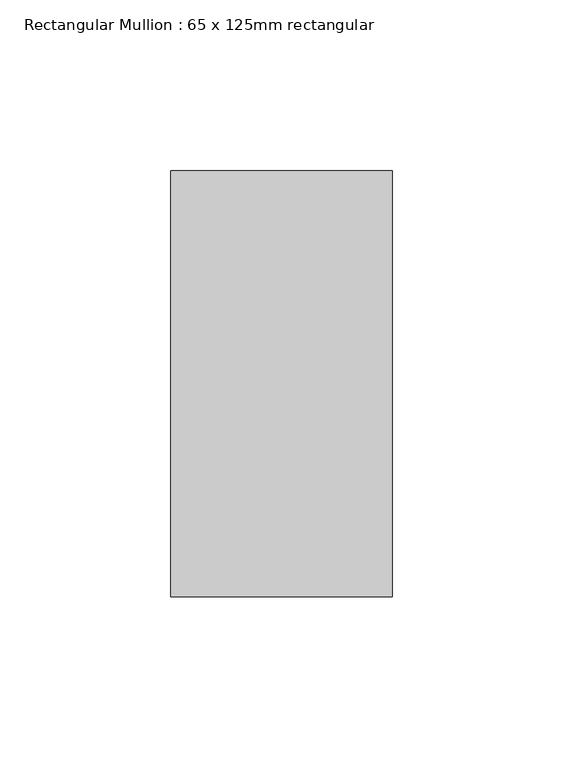
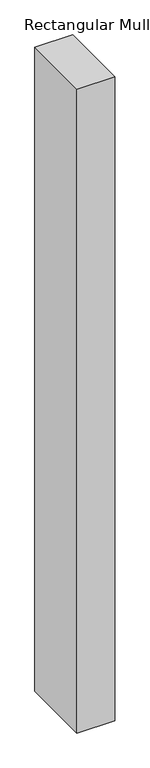
"""IFC4 building model written with IfcOpenShell, lengths in millimetres: member geometry, Rectangular Mullion : 65 x 125mm rectangular."""

from ifc_helpers import new_model, si_unit, frame, origin, place, context, project, spatial, polyline, outline, extrude, source, transform, mapped, element, save


def rectangular_mullion_65_x_125mm_rectangular_d33d7bb0(model_context):
    return source(origin(), model_context, "Body", "SweptSolid", [
        extrude(outline(polyline([(32.5, 62.5), (32.5, -62.5), (-32.5, -62.5), (-32.5, 62.5), (32.5, 62.5)])), frame((0.0, 0.0, -1170.0), z_axis=(0.0, 0.0, 1.0), x_axis=(1.0, 0.0, 0.0)), (0.0, 0.0, 1.0), 1170.0),
    ])


if __name__ == "__main__":
    model = new_model("IFC4")
    model_context = context("Model", 3, world=origin())
    ifc_project = project(units=[si_unit("LENGTHUNIT", "METRE", prefix="MILLI")], contexts=[model_context])
    site = spatial("IfcSite", under=ifc_project)
    building = spatial("IfcBuilding", under=site)
    placement = place(None, origin())
    rectangular_mullion_65_x_125mm_rectangular_shape = rectangular_mullion_65_x_125mm_rectangular_d33d7bb0(model_context)
    element("IfcMember", 1, ObjectType="Rectangular Mullion : 65 x 125mm rectangular", at=placement, inside=building, context=model_context, shape_type="MappedRepresentation", body=[
        mapped(rectangular_mullion_65_x_125mm_rectangular_shape, transform((0.0, 0.0, 0.0), x_axis=(1.0, 0.0, 0.0), y_axis=(0.0, 1.0, 0.0), z_axis=(0.0, 0.0, 1.0))),
    ])
    save(model, "model.ifc")

# Revit data of these elements
# Type "Rectangular Mullion : 65 x 125mm rectangular"
#   built-in parameter 1007304 = 0.410105 (stored number, unit not read)
#   built-in parameter 1007301 = 0.106627 (stored number, unit not read)
#   built-in parameter 1007300 = 0.106627 (stored number, unit not read)
# Element 1 (IfcMember, "Rectangular Mullion : 65 x 125mm rectangular")
#   Materials on its faces: "Aluminum"
# Materials
#   "Aluminum": class "Metal", colour RGB 244 245 246, transparency 0, Description = "Aluminum 6061", Cost = 0
